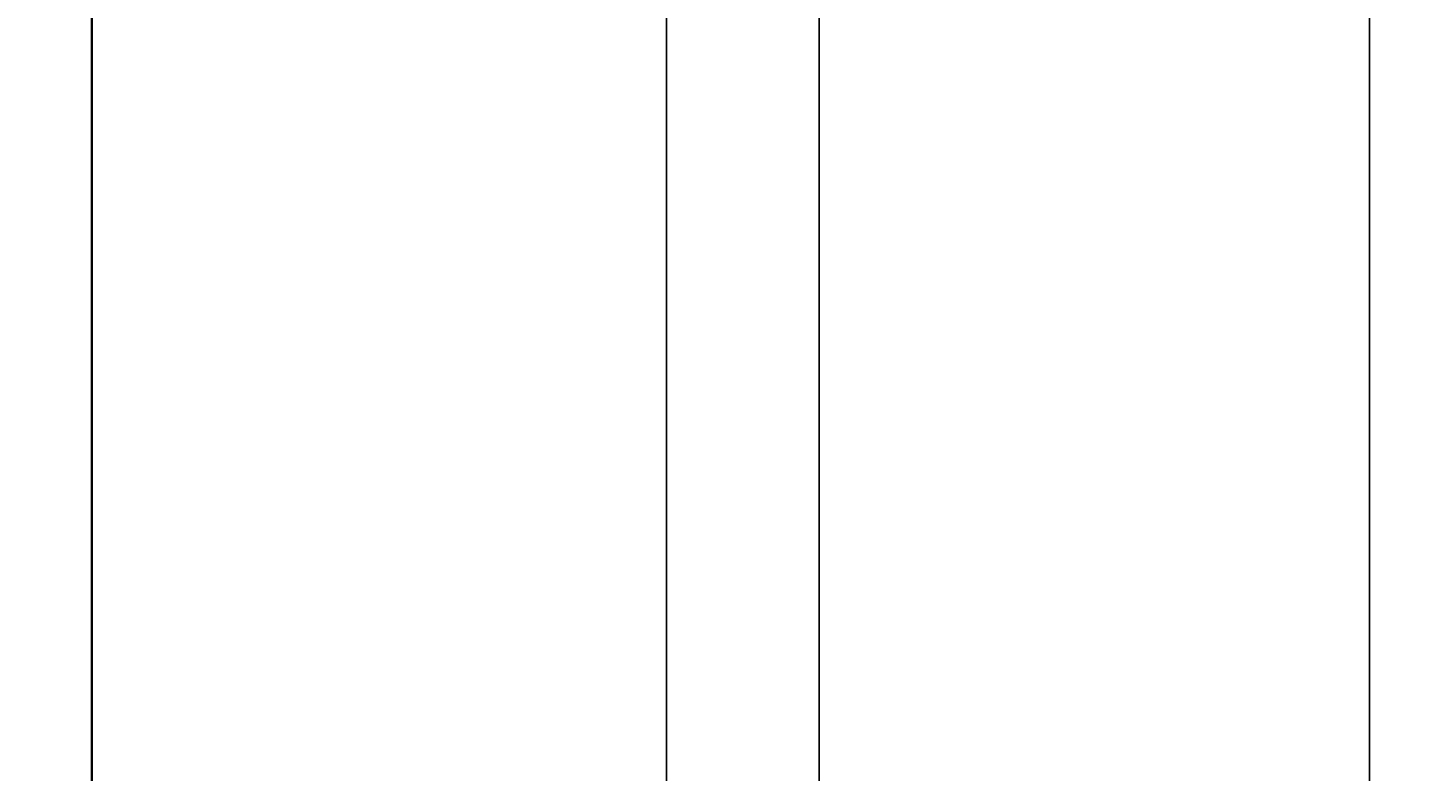
# Model space of a CAD drawing. Units: inches. Extents: x 738 to 1068, y 378 to 757.
# Tile 20 of 41: x 779 to 833, y 492 to 521. Entities that reach past the tile are written whole.
import ezdxf

# ---------------------------------------------------------------- set-up
doc = ezdxf.new("R2010")
doc.units = ezdxf.units.IN
doc.header["$MEASUREMENT"] = 0
doc.layers.add('A-ANNO-DIMS', color=2, linetype='Continuous', lineweight=18)
doc.layers.add('E-POWR-FEED', color=7, linetype='Continuous', lineweight=35)
doc.styles.get("Standard").update_dxf_attribs({"font": 'arial.ttf'})
doc.dimstyles.get("Standard").update_dxf_attribs({"dimtxt": 0.18, "dimasz": 0.18, "dimexe": 0.18, "dimexo": 0.0625, "dimgap": 0.09, "dimtad": 0, "dimtih": 1, "dimtoh": 1, "dimdec": 4, "dimzin": 0, "dimdsep": 46, "dimtxsty": 'Standard', "dimcen": 0.09, "dimadec": 0, "dimazin": 0, "dimtfac": 1, "dimtdec": 4, "dimtofl": 0, "dimtmove": 0, "dimatfit": 3, "dimfxl": 1, "dimtolj": 1, "dimtzin": 0, "dimarcsym": 0})

# ---------------------------------------------------------------- blocks, each defined once
blk = doc.blocks.new('*D21')
at = {"layer": 'A-ANNO-DIMS', "color": 0, "lineweight": -2, "transparency": 16777216}
for p, q in [((781.427, 531.401), (738.194, 531.401)), ((738.374, 531.221), (738.374, 496.578)), ((738.374, 461.572), (738.374, 496.215)), ((781.427, 461.392), (738.194, 461.392))]:
    blk.add_line(p, q, dxfattribs=at)
at = {"layer": 'A-ANNO-DIMS', "color": 0, "transparency": 16777216}
for points in [[(738.344, 531.221), (738.404, 531.221), (738.374, 531.401)], [(738.344, 461.572), (738.404, 461.572), (738.374, 461.392)]]:
    blk.add_solid(points, dxfattribs=at)
at = {"layer": 'Defpoints', "color": 0, "transparency": 16777216}
for p in [(738.374, 531.401), (781.49, 531.401), (781.49, 461.392)]:
    blk.add_point(p, dxfattribs=at)
at = {"layer": 'A-ANNO-DIMS', "color": 0, "transparency": 16777216, "insert": (738.374, 496.396), "char_height": 0.18, "attachment_point": 5}
blk.add_mtext('\\A1;70.01', dxfattribs=at)
blk = doc.blocks.new('*D25')
at = {"layer": 'A-ANNO-DIMS', "color": 0, "lineweight": -2, "transparency": 16777216}
for p, q in [((781.49, 646.923), (781.49, 378.239)), ((803.522, 646.923), (803.522, 378.239)), ((781.67, 378.419), (792.111, 378.419)), ((803.342, 378.419), (792.901, 378.419))]:
    blk.add_line(p, q, dxfattribs=at)
at = {"layer": 'A-ANNO-DIMS', "color": 0, "transparency": 16777216}
for points in [[(781.67, 378.449), (781.67, 378.389), (781.49, 378.419)], [(803.342, 378.449), (803.342, 378.389), (803.522, 378.419)]]:
    blk.add_solid(points, dxfattribs=at)
at = {"layer": 'Defpoints', "color": 0, "transparency": 16777216}
for p in [(781.49, 646.985), (803.522, 646.985), (803.522, 378.419)]:
    blk.add_point(p, dxfattribs=at)
at = {"layer": 'A-ANNO-DIMS', "color": 0, "transparency": 16777216, "insert": (792.506, 378.419), "char_height": 0.18, "attachment_point": 5}
blk.add_mtext('\\A1;22.03', dxfattribs=at)
blk = doc.blocks.new('*D32')
at = {"layer": 'A-ANNO-DIMS', "color": 0, "lineweight": -2, "transparency": 16777216}
for p, q in [((809.38, 461.454), (809.38, 756.505)), ((836.232, 461.277), (836.232, 756.505)), ((809.56, 756.325), (822.41, 756.325)), ((836.052, 756.325), (823.202, 756.325))]:
    blk.add_line(p, q, dxfattribs=at)
at = {"layer": 'A-ANNO-DIMS', "color": 0, "transparency": 16777216}
for points in [[(809.56, 756.355), (809.56, 756.295), (809.38, 756.325)], [(836.052, 756.355), (836.052, 756.295), (836.232, 756.325)]]:
    blk.add_solid(points, dxfattribs=at)
at = {"layer": 'Defpoints', "color": 0, "transparency": 16777216}
for p in [(836.232, 756.325), (809.38, 461.392), (836.232, 461.214)]:
    blk.add_point(p, dxfattribs=at)
at = {"layer": 'A-ANNO-DIMS', "color": 0, "transparency": 16777216, "insert": (822.806, 756.325), "char_height": 0.18, "attachment_point": 5}
blk.add_mtext('\\A1;26.85', dxfattribs=at)
blk = doc.blocks.new('*D34')
at = {"layer": 'A-ANNO-DIMS', "color": 0, "lineweight": -2, "transparency": 16777216}
for p, q in [((781.49, 686.266), (781.49, 378.239)), ((830.489, 686.266), (830.489, 378.239)), ((781.67, 378.419), (805.767, 378.419)), ((830.309, 378.419), (806.212, 378.419))]:
    blk.add_line(p, q, dxfattribs=at)
at = {"layer": 'A-ANNO-DIMS', "color": 0, "transparency": 16777216}
for points in [[(781.67, 378.449), (781.67, 378.389), (781.49, 378.419)], [(830.309, 378.449), (830.309, 378.389), (830.489, 378.419)]]:
    blk.add_solid(points, dxfattribs=at)
at = {"layer": 'Defpoints', "color": 0, "transparency": 16777216}
for p in [(781.49, 686.329), (830.489, 686.329), (830.489, 378.419)]:
    blk.add_point(p, dxfattribs=at)
at = {"layer": 'A-ANNO-DIMS', "color": 0, "transparency": 16777216, "insert": (805.99, 378.419), "char_height": 0.18, "attachment_point": 5}
blk.add_mtext('\\A1;49', dxfattribs=at)
blk = doc.blocks.new('*D38')
at = {"layer": 'A-ANNO-DIMS', "color": 0, "lineweight": -2, "transparency": 16777216}
for p, q in [((781.485, 593.017), (781.485, 378.239)), ((887.04, 593.067), (887.04, 378.239)), ((781.665, 378.419), (833.807, 378.419)), ((886.86, 378.419), (834.718, 378.419))]:
    blk.add_line(p, q, dxfattribs=at)
at = {"layer": 'A-ANNO-DIMS', "color": 0, "transparency": 16777216}
for points in [[(781.665, 378.449), (781.665, 378.389), (781.485, 378.419)], [(886.86, 378.449), (886.86, 378.389), (887.04, 378.419)]]:
    blk.add_solid(points, dxfattribs=at)
at = {"layer": 'Defpoints', "color": 0, "transparency": 16777216}
for p in [(781.485, 593.08), (887.04, 593.13), (887.04, 378.419)]:
    blk.add_point(p, dxfattribs=at)
at = {"layer": 'A-ANNO-DIMS', "color": 0, "transparency": 16777216, "insert": (834.263, 378.419), "char_height": 0.18, "attachment_point": 5}
blk.add_mtext('\\A1;105.56', dxfattribs=at)

msp = doc.modelspace()

# ---------------------------------------------------------------- linework, layer by layer
at = {"layer": 'E-POWR-FEED'}
msp.add_line((781.4897, 686.329), (781.4897, 437.7164), dxfattribs=at)

# ---------------------------------------------------------------- dimensions: what is measured, and where the dimension line sits
at = {"layer": 'A-ANNO-DIMS'}
for base, p1, p2, override, picture, middle in [((836.2324, 756.3251), (809.3803, 461.3919), (836.2324, 461.214), {"dimdec": 2, "dimlfac": 1, "dimrnd": 0, "dimzin": 0, "dimdsep": 46, "dimlunit": 2}, '*D32', (822.8064, 756.3251)), ((830.4893, 378.4191), (781.4897, 686.329), (830.4893, 686.329), {"dimdec": 0, "dimlfac": 1, "dimrnd": 0, "dimzin": 0, "dimdsep": 46, "dimlunit": 2}, '*D34', (805.9895, 378.4191)), ((803.5218, 378.4191), (781.4897, 646.9853), (803.5218, 646.9853), {"dimdec": 2, "dimlfac": 1, "dimrnd": 0, "dimzin": 0, "dimdsep": 46, "dimlunit": 2}, '*D25', (792.5057, 378.4191)), ((887.0404, 378.4191), (781.4846, 593.0796), (887.0404, 593.1296), {"dimdec": 2, "dimlfac": 1, "dimrnd": 0, "dimzin": 0, "dimdsep": 46, "dimlunit": 2}, '*D38', (834.2625, 378.4191))]:
    dim = msp.add_linear_dim(base=base, p1=p1, p2=p2, dimstyle='Standard', override=override, dxfattribs=at)
    dim.commit()
    dim.dimension.update_dxf_attribs({"geometry": picture, "text_midpoint": middle})
dim = msp.add_linear_dim(base=(738.3736, 531.4009), p1=(781.4897, 461.3919), p2=(781.4897, 531.4009), angle=90, dimstyle='Standard', override={"dimdec": 2, "dimlfac": 1, "dimrnd": 0, "dimzin": 0, "dimdsep": 46, "dimlunit": 2}, dxfattribs=at)
dim.commit()
dim.dimension.update_dxf_attribs({"geometry": '*D21', "text_midpoint": (738.3736, 496.3964)})

doc.saveas('drawing.dxf')
